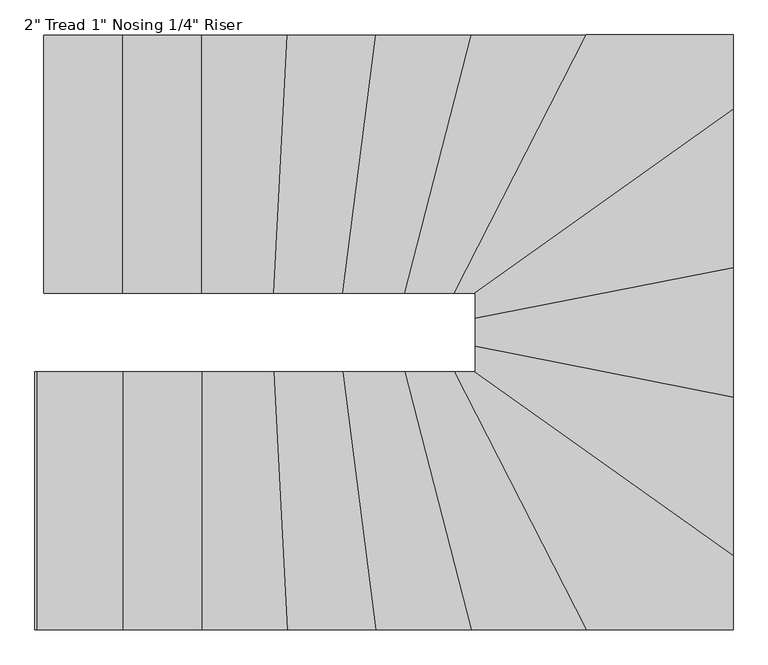
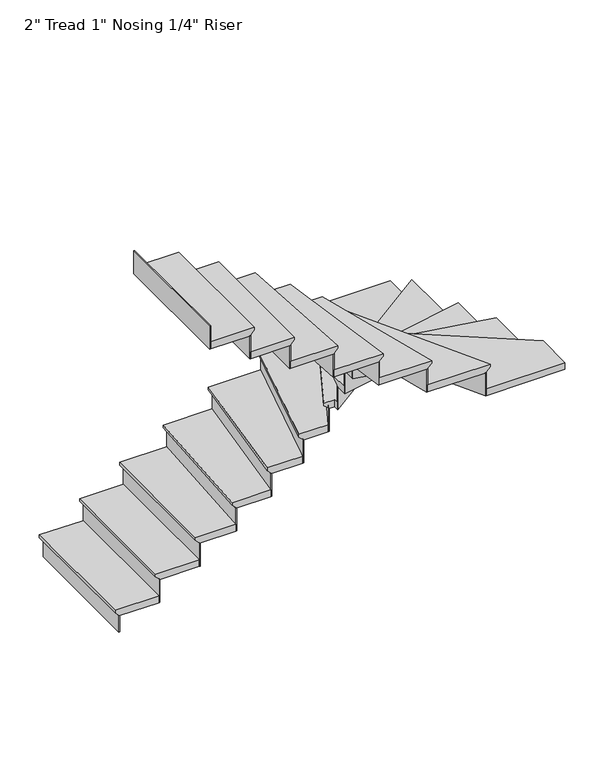
"""IFC4 building model written with IfcOpenShell, lengths in millimetres: stair flight geometry."""

from ifc_helpers import new_model, si_unit, origin, place, context, project, spatial, faceted_brep, source, transform, mapped, element, save


def stair_flight_b9c50625(model_context):
    return source(origin(), model_context, "Body", "Brep", [
        faceted_brep([(1342.8282136, -2159.7365003, 3350.6833333), (1342.8282136, -2159.7365003, 3369.7333333), (1342.8282136, -1245.3365003, 3369.7333333), (1342.8282136, -1245.3365003, 3350.6833333), (1368.2282136, -2159.7365003, 3325.2833333), (1368.2282136, -1245.3365003, 3325.2833333), (1647.6282136, -2159.7365003, 3369.7333333), (1647.6282136, -1245.3365003, 3369.7333333), (1368.2282136, -1245.3365003, 3318.9333333), (1647.6282136, -1245.3365003, 3318.9333333), (1647.6282136, -2159.7365003, 3318.9333333), (1368.2282136, -2159.7365003, 3318.9333333)], [[[0, 1, 2, 3]], [[4, 0, 3, 5]], [[2, 1, 6, 7]], [[8, 9, 10, 11]], [[2, 7, 9, 8, 5, 3]], [[8, 11, 4, 5]], [[6, 1, 0, 4, 11, 10]], [[7, 6, 10, 9]]]),
        faceted_brep([(1368.2282136, -2159.7365003, 3318.9333333), (1368.2282136, -2159.7365003, 3200.4), (1374.5782136, -2159.7365003, 3200.4), (1374.5782136, -2159.7365003, 3318.9333333), (1368.2282136, -1245.3365003, 3318.9333333), (1374.5782136, -1245.3365003, 3318.9333333), (1374.5782136, -1245.3365003, 3200.4), (1368.2282136, -1245.3365003, 3200.4)], [[[0, 1, 2, 3]], [[4, 5, 6, 7]], [[1, 0, 4, 7]], [[2, 1, 7, 6]], [[3, 2, 6, 5]], [[0, 3, 5, 4]]]),
        faceted_brep([(1647.6282136, -2159.7365003, 3488.2666667), (1647.6282136, -2159.7365003, 3318.9333333), (1653.9782136, -2159.7365003, 3318.9333333), (1653.9782136, -2159.7365003, 3488.2666667), (1647.6282136, -1245.3365003, 3488.2666667), (1653.9782136, -1245.3365003, 3488.2666667), (1653.9782136, -1245.3365003, 3318.9333333), (1647.6282136, -1245.3365003, 3318.9333333)], [[[0, 1, 2, 3]], [[4, 5, 6, 7]], [[1, 0, 4, 7]], [[2, 1, 7, 6]], [[3, 2, 6, 5]], [[0, 3, 5, 4]]]),
        faceted_brep([(1622.2282136, -1245.3365003, 3539.0666667), (1622.2282136, -2159.7365003, 3539.0666667), (1927.0282136, -2159.7365003, 3539.0666667), (1927.0282136, -1245.3365003, 3539.0666667), (1647.6282136, -1245.3365003, 3488.2666667), (1927.0282136, -1245.3365003, 3488.2666667), (1927.0282136, -2159.7365003, 3488.2666667), (1647.6282136, -2159.7365003, 3488.2666667), (1647.6282136, -1245.3365003, 3494.6166667), (1622.2282136, -1245.3365003, 3520.0166667), (1647.6282136, -2159.7365003, 3494.6166667), (1622.2282136, -2159.7365003, 3520.0166667)], [[[0, 1, 2, 3]], [[4, 5, 6, 7]], [[0, 3, 5, 4, 8, 9]], [[4, 7, 10, 8]], [[2, 1, 11, 10, 7, 6]], [[3, 2, 6, 5]], [[11, 1, 0, 9]], [[10, 11, 9, 8]]]),
        faceted_brep([(1927.0282136, -2159.7365003, 3657.6), (1927.0282136, -2159.7365003, 3488.2666667), (1933.3782136, -2159.7365003, 3488.2666667), (1933.3782136, -2159.7365003, 3657.6), (1927.0282136, -1245.3365003, 3657.6), (1933.3782136, -1245.3365003, 3657.6), (1933.3782136, -1245.3365003, 3488.2666667), (1927.0282136, -1245.3365003, 3488.2666667)], [[[0, 1, 2, 3]], [[4, 5, 6, 7]], [[1, 0, 4, 7]], [[2, 1, 7, 6]], [[3, 2, 6, 5]], [[0, 3, 5, 4]]]),
        faceted_brep([(1901.6282136, -1245.3365003, 3708.4), (1901.6282136, -2159.7365003, 3708.4), (2182.6953751, -2159.7365003, 3708.4), (2230.2296455, -1245.3365003, 3708.4), (1927.0282136, -1245.3365003, 3657.6), (2230.2296455, -1245.3365003, 3657.6), (2182.6953751, -2159.7365003, 3657.6), (1927.0282136, -2159.7365003, 3657.6), (1927.0282136, -1245.3365003, 3663.95), (1901.6282136, -1245.3365003, 3689.35), (1927.0282136, -2159.7365003, 3663.95), (1901.6282136, -2159.7365003, 3689.35)], [[[0, 1, 2, 3]], [[4, 5, 6, 7]], [[0, 3, 5, 4, 8, 9]], [[4, 7, 10, 8]], [[2, 1, 11, 10, 7, 6]], [[3, 2, 6, 5]], [[11, 1, 0, 9]], [[10, 11, 9, 8]]]),
        faceted_brep([(2182.6953751, -2159.7365003, 3826.9333333), (2182.6953751, -2159.7365003, 3657.6), (2189.0539493, -2159.7365003, 3657.6), (2189.0539493, -2159.7365003, 3826.9333333), (2230.2296455, -1245.3365003, 3826.9333333), (2236.5882197, -1245.3365003, 3826.9333333), (2236.5882197, -1245.3365003, 3657.6), (2230.2296455, -1245.3365003, 3657.6)], [[[0, 1, 2, 3]], [[4, 5, 6, 7]], [[1, 0, 4, 7]], [[2, 1, 7, 6]], [[3, 2, 6, 5]], [[0, 3, 5, 4]]]),
        faceted_brep([(2204.7953488, -1245.3365003, 3877.7333333), (2157.2610784, -2159.7365003, 3877.7333333), (2426.8620749, -2159.7365003, 3877.7333333), (2545.2181266, -1245.3365003, 3877.7333333), (2230.2296455, -1245.3365003, 3826.9333333), (2545.2181266, -1245.3365003, 3826.9333333), (2426.8620749, -2159.7365003, 3826.9333333), (2182.6953751, -2159.7365003, 3826.9333333), (2230.2296455, -1245.3365003, 3833.2833333), (2204.7953488, -1245.3365003, 3858.6833333), (2182.6953751, -2159.7365003, 3833.2833333), (2157.2610784, -2159.7365003, 3858.6833333)], [[[0, 1, 2, 3]], [[4, 5, 6, 7]], [[0, 3, 5, 4, 8, 9]], [[4, 7, 10, 8]], [[2, 1, 11, 10, 7, 6]], [[3, 2, 6, 5]], [[11, 1, 0, 9]], [[10, 11, 9, 8]]]),
        faceted_brep([(2426.8620749, -2159.7365003, 3996.2666667), (2426.8620749, -2159.7365003, 3826.9333333), (2433.2650467, -2159.7365003, 3826.9333333), (2433.2650467, -2159.7365003, 3996.2666667), (2545.2181266, -1245.3365003, 3996.2666667), (2551.6210984, -1245.3365003, 3996.2666667), (2551.6210984, -1245.3365003, 3826.9333333), (2545.2181266, -1245.3365003, 3826.9333333)], [[[0, 1, 2, 3]], [[4, 5, 6, 7]], [[1, 0, 4, 7]], [[2, 1, 7, 6]], [[3, 2, 6, 5]], [[0, 3, 5, 4]]]),
        faceted_brep([(2519.6062395, -1245.3365003, 4047.0666667), (2401.2501878, -2159.7365003, 4047.0666667), (2648.4892974, -2159.7365003, 4047.0666667), (2883.6197448, -1245.3365003, 4047.0666667), (2545.2181266, -1245.3365003, 3996.2666667), (2883.6197448, -1245.3365003, 3996.2666667), (2648.4892974, -2159.7365003, 3996.2666667), (2426.8620749, -2159.7365003, 3996.2666667), (2545.2181266, -1245.3365003, 4002.6166667), (2519.6062395, -1245.3365003, 4028.0166667), (2426.8620749, -2159.7365003, 4002.6166667), (2401.2501878, -2159.7365003, 4028.0166667)], [[[0, 1, 2, 3]], [[4, 5, 6, 7]], [[0, 3, 5, 4, 8, 9]], [[4, 7, 10, 8]], [[2, 1, 11, 10, 7, 6]], [[3, 2, 6, 5]], [[11, 1, 0, 9]], [[10, 11, 9, 8]]]),
        faceted_brep([(2648.4892974, -2159.7365003, 4165.6), (2648.4892974, -2159.7365003, 3996.2666667), (2655.0458743, -2159.7365003, 3996.2666667), (2655.0458743, -2159.7365003, 4165.6), (2883.6197448, -1245.3365003, 4165.6), (2890.1763217, -1245.3365003, 4165.6), (2890.1763217, -1245.3365003, 3996.2666667), (2883.6197448, -1245.3365003, 3996.2666667)], [[[0, 1, 2, 3]], [[4, 5, 6, 7]], [[1, 0, 4, 7]], [[2, 1, 7, 6]], [[3, 2, 6, 5]], [[0, 3, 5, 4]]]),
        faceted_brep([(2857.3934373, -1245.3365003, 4216.4), (2622.2629899, -2159.7365003, 4216.4), (2824.8359335, -2159.7365003, 4216.4), (3293.6605548, -1245.3365003, 4216.4), (2883.6197448, -1245.3365003, 4165.6), (3293.6605548, -1245.3365003, 4165.6), (2824.8359335, -2159.7365003, 4165.6), (2648.4892974, -2159.7365003, 4165.6), (2883.6197448, -1245.3365003, 4171.95), (2857.3934373, -1245.3365003, 4197.35), (2648.4892974, -2159.7365003, 4171.95), (2622.2629899, -2159.7365003, 4197.35)], [[[0, 1, 2, 3]], [[4, 5, 6, 7]], [[0, 3, 5, 4, 8, 9]], [[4, 7, 10, 8]], [[2, 1, 11, 10, 7, 6]], [[3, 2, 6, 5]], [[11, 1, 0, 9]], [[10, 11, 9, 8]]]),
        faceted_brep([(2824.8359335, -2159.7365003, 4334.9333333), (2824.8359335, -2159.7365003, 4165.6), (2831.9719166, -2159.7365003, 4165.6), (2831.9719166, -2159.7365003, 4334.9333333), (3293.6605548, -1245.3365003, 4334.9333333), (3300.7965379, -1245.3365003, 4334.9333333), (3300.7965379, -1245.3365003, 4165.6), (3293.6605548, -1245.3365003, 4165.6)], [[[0, 1, 2, 3]], [[4, 5, 6, 7]], [[1, 0, 4, 7]], [[2, 1, 7, 6]], [[3, 2, 6, 5]], [[0, 3, 5, 4]]]),
        faceted_brep([(3784.9599055, -1539.017634, 4385.7333333), (3784.9599055, -1245.3365003, 4385.7333333), (3265.1166223, -1245.3365003, 4385.7333333), (2796.2920009, -2159.7365003, 4385.7333333), (2870.5599055, -2159.7365003, 4385.7333333), (2870.5599055, -2189.2915832, 4385.7333333), (3784.9599055, -1245.3365003, 4334.9333333), (3784.9599055, -1539.017634, 4334.9333333), (2870.5599055, -2189.2915832, 4334.9333333), (2870.5599055, -2159.7365003, 4334.9333333), (2824.8359335, -2159.7365003, 4334.9333333), (3293.6605548, -1245.3365003, 4334.9333333), (3293.6605548, -1245.3365003, 4341.2833333), (3265.1166223, -1245.3365003, 4366.6833333), (2824.8359335, -2159.7365003, 4341.2833333), (2796.2920009, -2159.7365003, 4366.6833333)], [[[0, 1, 2, 3, 4, 5]], [[6, 7, 8, 9, 10, 11]], [[1, 0, 7, 6]], [[2, 1, 6, 11, 12, 13]], [[11, 10, 14, 12]], [[4, 3, 15, 14, 10, 9]], [[5, 4, 9, 8]], [[0, 5, 8, 7]], [[15, 3, 2, 13]], [[14, 15, 13, 12]]]),
        faceted_brep([(2870.5599055, -2189.2915832, 4504.2666667), (2870.5599055, -2189.2915832, 4334.9333333), (2870.5599055, -2197.083558, 4334.9333333), (2870.5599055, -2197.083558, 4504.2666667), (3784.9599055, -1539.017634, 4504.2666667), (3784.9599055, -1546.8096088, 4504.2666667), (3784.9599055, -1546.8096088, 4334.9333333), (3784.9599055, -1539.017634, 4334.9333333)], [[[0, 1, 2, 3]], [[4, 5, 6, 7]], [[1, 0, 4, 7]], [[2, 1, 7, 6]], [[3, 2, 6, 5]], [[0, 3, 5, 4]]]),
        faceted_brep([(3784.9599055, -1507.8497349, 4555.0666667), (2870.5599055, -2158.123684, 4555.0666667), (2870.5599055, -2275.7456703, 4555.0666667), (3784.9599055, -2095.5048139, 4555.0666667), (3784.9599055, -1539.017634, 4504.2666667), (3784.9599055, -2095.5048139, 4504.2666667), (2870.5599055, -2275.7456703, 4504.2666667), (2870.5599055, -2189.2915832, 4504.2666667), (3784.9599055, -1539.017634, 4510.6166667), (3784.9599055, -1507.8497349, 4536.0166667), (2870.5599055, -2189.2915832, 4510.6166667), (2870.5599055, -2158.123684, 4536.0166667)], [[[0, 1, 2, 3]], [[4, 5, 6, 7]], [[0, 3, 5, 4, 8, 9]], [[4, 7, 10, 8]], [[2, 1, 11, 10, 7, 6]], [[3, 2, 6, 5]], [[11, 1, 0, 9]], [[10, 11, 9, 8]]]),
        faceted_brep([(2870.5599055, -2275.7456703, 4673.6), (2870.5599055, -2275.7456703, 4504.2666667), (2870.5599055, -2282.2178557, 4504.2666667), (2870.5599055, -2282.2178557, 4673.6), (3784.9599055, -2095.5048139, 4673.6), (3784.9599055, -2101.9769994, 4673.6), (3784.9599055, -2101.9769994, 4504.2666667), (3784.9599055, -2095.5048139, 4504.2666667)], [[[0, 1, 2, 3]], [[4, 5, 6, 7]], [[1, 0, 4, 7]], [[2, 1, 7, 6]], [[3, 2, 6, 5]], [[0, 3, 5, 4]]]),
        faceted_brep([(3784.9599055, -2069.6160722, 4724.4), (2870.5599055, -2249.8569285, 4724.4), (2870.5599055, -2374.9048139, 4724.4), (3784.9599055, -2555.1456703, 4724.4), (3784.9599055, -2095.5048139, 4673.6), (3784.9599055, -2555.1456703, 4673.6), (2870.5599055, -2374.9048139, 4673.6), (2870.5599055, -2275.7456703, 4673.6), (3784.9599055, -2095.5048139, 4679.95), (3784.9599055, -2069.6160722, 4705.35), (2870.5599055, -2275.7456703, 4679.95), (2870.5599055, -2249.8569285, 4705.35)], [[[0, 1, 2, 3]], [[4, 5, 6, 7]], [[0, 3, 5, 4, 8, 9]], [[4, 7, 10, 8]], [[2, 1, 11, 10, 7, 6]], [[3, 2, 6, 5]], [[11, 1, 0, 9]], [[10, 11, 9, 8]]]),
        faceted_brep([(2870.5599055, -2374.9048139, 4842.9333333), (2870.5599055, -2374.9048139, 4673.6), (2870.5599055, -2381.3769994, 4673.6), (2870.5599055, -2381.3769994, 4842.9333333), (3784.9599055, -2555.1456703, 4842.9333333), (3784.9599055, -2561.6178557, 4842.9333333), (3784.9599055, -2561.6178557, 4673.6), (3784.9599055, -2555.1456703, 4673.6)], [[[0, 1, 2, 3]], [[4, 5, 6, 7]], [[1, 0, 4, 7]], [[2, 1, 7, 6]], [[3, 2, 6, 5]], [[0, 3, 5, 4]]]),
        faceted_brep([(3784.9599055, -2529.2569285, 4893.7333333), (2870.5599055, -2349.0160722, 4893.7333333), (2870.5599055, -2439.1365003, 4893.7333333), (2824.464431, -2439.1365003, 4893.7333333), (3784.9599055, -3122.191165, 4893.7333333), (3784.9599055, -2555.1456703, 4842.9333333), (3784.9599055, -3122.191165, 4842.9333333), (2824.464431, -2439.1365003, 4842.9333333), (2870.5599055, -2439.1365003, 4842.9333333), (2870.5599055, -2374.9048139, 4842.9333333), (3784.9599055, -2555.1456703, 4849.2833333), (3784.9599055, -2529.2569285, 4874.6833333), (2870.5599055, -2374.9048139, 4849.2833333), (2870.5599055, -2349.0160722, 4874.6833333)], [[[0, 1, 2, 3, 4]], [[5, 6, 7, 8, 9]], [[0, 4, 6, 5, 10, 11]], [[5, 9, 12, 10]], [[2, 1, 13, 12, 9, 8]], [[3, 2, 8, 7]], [[4, 3, 7, 6]], [[13, 1, 0, 11]], [[12, 13, 11, 10]]]),
        faceted_brep([(2824.464431, -2439.1365003, 5012.2666667), (2824.464431, -2439.1365003, 4842.9333333), (2813.5075385, -2439.1365003, 4842.9333333), (2813.5075385, -2439.1365003, 5012.2666667), (3784.9599055, -3122.191165, 5012.2666667), (3784.9599055, -3129.9831398, 5012.2666667), (3784.9599055, -3129.9831398, 4842.9333333), (3784.9599055, -3122.191165, 4842.9333333)], [[[0, 1, 2, 3]], [[4, 5, 6, 7]], [[1, 0, 4, 7]], [[2, 1, 7, 6]], [[3, 2, 6, 5]], [[0, 3, 5, 4]]]),
        faceted_brep([(3236.5726897, -3353.5365003, 5063.0666667), (3784.9599055, -3353.5365003, 5063.0666667), (3784.9599055, -3091.0232658, 5063.0666667), (2868.2920009, -2439.1365003, 5063.0666667), (2767.7480684, -2439.1365003, 5063.0666667), (3784.9599055, -3353.5365003, 5012.2666667), (3236.5726897, -3353.5365003, 5012.2666667), (2767.7480684, -2439.1365003, 5012.2666667), (2824.464431, -2439.1365003, 5012.2666667), (3784.9599055, -3122.191165, 5012.2666667), (3784.9599055, -3122.191165, 5018.6166667), (3784.9599055, -3091.0232658, 5044.0166667), (2824.464431, -2439.1365003, 5018.6166667), (2868.2920009, -2439.1365003, 5044.0166667)], [[[0, 1, 2, 3, 4]], [[5, 6, 7, 8, 9]], [[1, 0, 6, 5]], [[2, 1, 5, 9, 10, 11]], [[9, 8, 12, 10]], [[4, 3, 13, 12, 8, 7]], [[0, 4, 7, 6]], [[13, 3, 2, 11]], [[12, 13, 11, 10]]]),
        faceted_brep([(2767.7480684, -2439.1365003, 5181.6), (2767.7480684, -2439.1365003, 5012.2666667), (2760.6120853, -2439.1365003, 5012.2666667), (2760.6120853, -2439.1365003, 5181.6), (3236.5726897, -3353.5365003, 5181.6), (3229.4367066, -3353.5365003, 5181.6), (3229.4367066, -3353.5365003, 5012.2666667), (3236.5726897, -3353.5365003, 5012.2666667)], [[[0, 1, 2, 3]], [[4, 5, 6, 7]], [[1, 0, 4, 7]], [[2, 1, 7, 6]], [[3, 2, 6, 5]], [[0, 3, 5, 4]]]),
        faceted_brep([(3265.1166223, -3353.5365003, 5232.4), (2796.2920009, -2439.1365003, 5232.4), (2596.0366825, -2439.1365003, 5232.4), (2831.1671299, -3353.5365003, 5232.4), (3236.5726897, -3353.5365003, 5181.6), (2831.1671299, -3353.5365003, 5181.6), (2596.0366825, -2439.1365003, 5181.6), (2767.7480684, -2439.1365003, 5181.6), (3236.5726897, -3353.5365003, 5187.95), (3265.1166223, -3353.5365003, 5213.35), (2767.7480684, -2439.1365003, 5187.95), (2796.2920009, -2439.1365003, 5213.35)], [[[0, 1, 2, 3]], [[4, 5, 6, 7]], [[0, 3, 5, 4, 8, 9]], [[4, 7, 10, 8]], [[2, 1, 11, 10, 7, 6]], [[3, 2, 6, 5]], [[11, 1, 0, 9]], [[10, 11, 9, 8]]]),
        faceted_brep([(2596.0366825, -2439.1365003, 5350.9333333), (2596.0366825, -2439.1365003, 5181.6), (2589.4801056, -2439.1365003, 5181.6), (2589.4801056, -2439.1365003, 5350.9333333), (2831.1671299, -3353.5365003, 5350.9333333), (2824.610553, -3353.5365003, 5350.9333333), (2824.610553, -3353.5365003, 5181.6), (2831.1671299, -3353.5365003, 5181.6)], [[[0, 1, 2, 3]], [[4, 5, 6, 7]], [[1, 0, 4, 7]], [[2, 1, 7, 6]], [[3, 2, 6, 5]], [[0, 3, 5, 4]]]),
        faceted_brep([(2857.3934373, -3353.5365003, 5401.7333333), (2622.2629899, -2439.1365003, 5401.7333333), (2375.6383007, -2439.1365003, 5401.7333333), (2493.9943524, -3353.5365003, 5401.7333333), (2831.1671299, -3353.5365003, 5350.9333333), (2493.9943524, -3353.5365003, 5350.9333333), (2375.6383007, -2439.1365003, 5350.9333333), (2596.0366825, -2439.1365003, 5350.9333333), (2831.1671299, -3353.5365003, 5357.2833333), (2857.3934373, -3353.5365003, 5382.6833333), (2596.0366825, -2439.1365003, 5357.2833333), (2622.2629899, -2439.1365003, 5382.6833333)], [[[0, 1, 2, 3]], [[4, 5, 6, 7]], [[0, 3, 5, 4, 8, 9]], [[4, 7, 10, 8]], [[2, 1, 11, 10, 7, 6]], [[3, 2, 6, 5]], [[11, 1, 0, 9]], [[10, 11, 9, 8]]]),
        faceted_brep([(2375.6383007, -2439.1365003, 5520.2666667), (2375.6383007, -2439.1365003, 5350.9333333), (2369.2353289, -2439.1365003, 5350.9333333), (2369.2353289, -2439.1365003, 5520.2666667), (2493.9943524, -3353.5365003, 5520.2666667), (2487.5913806, -3353.5365003, 5520.2666667), (2487.5913806, -3353.5365003, 5350.9333333), (2493.9943524, -3353.5365003, 5350.9333333)], [[[0, 1, 2, 3]], [[4, 5, 6, 7]], [[1, 0, 4, 7]], [[2, 1, 7, 6]], [[3, 2, 6, 5]], [[0, 3, 5, 4]]]),
        faceted_brep([(2519.6062395, -3353.5365003, 5571.0666667), (2401.2501878, -2439.1365003, 5571.0666667), (2131.8267818, -2439.1365003, 5571.0666667), (2179.3610522, -3353.5365003, 5571.0666667), (2493.9943524, -3353.5365003, 5520.2666667), (2179.3610522, -3353.5365003, 5520.2666667), (2131.8267818, -2439.1365003, 5520.2666667), (2375.6383007, -2439.1365003, 5520.2666667), (2493.9943524, -3353.5365003, 5526.6166667), (2519.6062395, -3353.5365003, 5552.0166667), (2375.6383007, -2439.1365003, 5526.6166667), (2401.2501878, -2439.1365003, 5552.0166667)], [[[0, 1, 2, 3]], [[4, 5, 6, 7]], [[0, 3, 5, 4, 8, 9]], [[4, 7, 10, 8]], [[2, 1, 11, 10, 7, 6]], [[3, 2, 6, 5]], [[11, 1, 0, 9]], [[10, 11, 9, 8]]]),
        faceted_brep([(2131.8267818, -2439.1365003, 5689.6), (2131.8267818, -2439.1365003, 5520.2666667), (2125.4682076, -2439.1365003, 5520.2666667), (2125.4682076, -2439.1365003, 5689.6), (2179.3610522, -3353.5365003, 5689.6), (2173.002478, -3353.5365003, 5689.6), (2173.002478, -3353.5365003, 5520.2666667), (2179.3610522, -3353.5365003, 5520.2666667)], [[[0, 1, 2, 3]], [[4, 5, 6, 7]], [[1, 0, 4, 7]], [[2, 1, 7, 6]], [[3, 2, 6, 5]], [[0, 3, 5, 4]]]),
        faceted_brep([(2204.7953488, -3353.5365003, 5740.4), (2157.2610784, -2439.1365003, 5740.4), (1876.2282136, -2439.1365003, 5740.4), (1876.2282136, -3353.5365003, 5740.4), (2179.3610522, -3353.5365003, 5689.6), (1876.2282136, -3353.5365003, 5689.6), (1876.2282136, -2439.1365003, 5689.6), (2131.8267818, -2439.1365003, 5689.6), (2179.3610522, -3353.5365003, 5695.95), (2204.7953488, -3353.5365003, 5721.35), (2131.8267818, -2439.1365003, 5695.95), (2157.2610784, -2439.1365003, 5721.35)], [[[0, 1, 2, 3]], [[4, 5, 6, 7]], [[0, 3, 5, 4, 8, 9]], [[4, 7, 10, 8]], [[2, 1, 11, 10, 7, 6]], [[3, 2, 6, 5]], [[11, 1, 0, 9]], [[10, 11, 9, 8]]]),
        faceted_brep([(1876.2282136, -2439.1365003, 5858.9333333), (1876.2282136, -2439.1365003, 5689.6), (1869.8782136, -2439.1365003, 5689.6), (1869.8782136, -2439.1365003, 5858.9333333), (1876.2282136, -3353.5365003, 5858.9333333), (1869.8782136, -3353.5365003, 5858.9333333), (1869.8782136, -3353.5365003, 5689.6), (1876.2282136, -3353.5365003, 5689.6)], [[[0, 1, 2, 3]], [[4, 5, 6, 7]], [[1, 0, 4, 7]], [[2, 1, 7, 6]], [[3, 2, 6, 5]], [[0, 3, 5, 4]]]),
        faceted_brep([(1901.6282136, -3353.5365003, 5909.7333333), (1901.6282136, -2439.1365003, 5909.7333333), (1596.8282136, -2439.1365003, 5909.7333333), (1596.8282136, -3353.5365003, 5909.7333333), (1876.2282136, -3353.5365003, 5858.9333333), (1596.8282136, -3353.5365003, 5858.9333333), (1596.8282136, -2439.1365003, 5858.9333333), (1876.2282136, -2439.1365003, 5858.9333333), (1876.2282136, -3353.5365003, 5865.2833333), (1901.6282136, -3353.5365003, 5890.6833333), (1876.2282136, -2439.1365003, 5865.2833333), (1901.6282136, -2439.1365003, 5890.6833333)], [[[0, 1, 2, 3]], [[4, 5, 6, 7]], [[0, 3, 5, 4, 8, 9]], [[4, 7, 10, 8]], [[2, 1, 11, 10, 7, 6]], [[3, 2, 6, 5]], [[11, 1, 0, 9]], [[10, 11, 9, 8]]]),
        faceted_brep([(1596.8282136, -2439.1365003, 6028.2666667), (1596.8282136, -2439.1365003, 5858.9333333), (1590.4782136, -2439.1365003, 5858.9333333), (1590.4782136, -2439.1365003, 6028.2666667), (1596.8282136, -3353.5365003, 6028.2666667), (1590.4782136, -3353.5365003, 6028.2666667), (1590.4782136, -3353.5365003, 5858.9333333), (1596.8282136, -3353.5365003, 5858.9333333)], [[[0, 1, 2, 3]], [[4, 5, 6, 7]], [[1, 0, 4, 7]], [[2, 1, 7, 6]], [[3, 2, 6, 5]], [[0, 3, 5, 4]]]),
        faceted_brep([(1317.4282136, -2439.1365003, 6197.6), (1317.4282136, -2439.1365003, 6028.2666667), (1311.0782136, -2439.1365003, 6028.2666667), (1311.0782136, -2439.1365003, 6197.6), (1317.4282136, -3353.5365003, 6197.6), (1311.0782136, -3353.5365003, 6197.6), (1311.0782136, -3353.5365003, 6028.2666667), (1317.4282136, -3353.5365003, 6028.2666667)], [[[0, 1, 2, 3]], [[4, 5, 6, 7]], [[1, 0, 4, 7]], [[2, 1, 7, 6]], [[3, 2, 6, 5]], [[0, 3, 5, 4]]]),
        faceted_brep([(1622.2282136, -3353.5365003, 6079.0666667), (1622.2282136, -2439.1365003, 6079.0666667), (1317.4282136, -2439.1365003, 6079.0666667), (1317.4282136, -3353.5365003, 6079.0666667), (1596.8282136, -3353.5365003, 6028.2666667), (1317.4282136, -3353.5365003, 6028.2666667), (1317.4282136, -2439.1365003, 6028.2666667), (1596.8282136, -2439.1365003, 6028.2666667), (1596.8282136, -3353.5365003, 6034.6166667), (1622.2282136, -3353.5365003, 6060.0166667), (1596.8282136, -2439.1365003, 6034.6166667), (1622.2282136, -2439.1365003, 6060.0166667)], [[[0, 1, 2, 3]], [[4, 5, 6, 7]], [[0, 3, 5, 4, 8, 9]], [[4, 7, 10, 8]], [[2, 1, 11, 10, 7, 6]], [[3, 2, 6, 5]], [[11, 1, 0, 9]], [[10, 11, 9, 8]]]),
    ])


if __name__ == "__main__":
    model = new_model("IFC4")
    model_context = context("Model", 3, world=origin())
    ifc_project = project(units=[si_unit("LENGTHUNIT", "METRE", prefix="MILLI")], contexts=[model_context])
    site = spatial("IfcSite", under=ifc_project)
    building = spatial("IfcBuilding", under=site)
    placement = place(None, origin())
    stair_flight_shape = stair_flight_b9c50625(model_context)
    element("IfcStairFlight", 1, ObjectType="2\" Tread 1\" Nosing 1/4\" Riser", at=placement, inside=building, context=model_context, shape_type="MappedRepresentation", body=[
        mapped(stair_flight_shape, transform((0.0, 0.0, 0.0), x_axis=(1.0, 0.0, 0.0), y_axis=(0.0, 1.0, 0.0), z_axis=(0.0, 0.0, 1.0))),
    ])
    save(model, "model.ifc")
